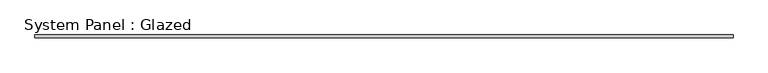
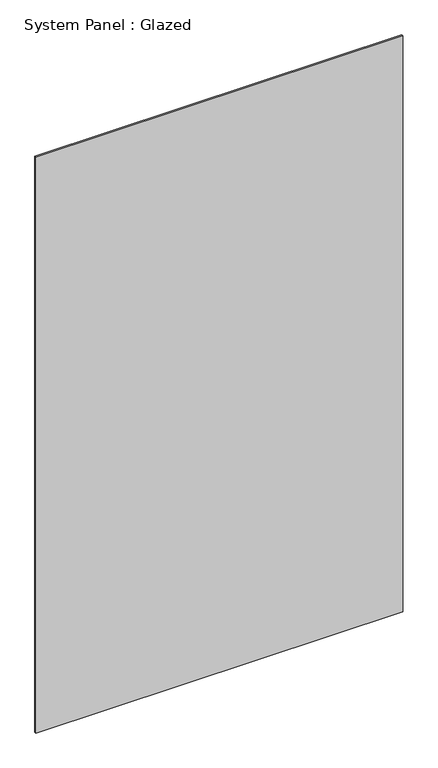
"""IFC4 building model written with IfcOpenShell, lengths in millimetres: plate geometry, System Panel : Glazed."""

from ifc_helpers import new_model, si_unit, origin, origin_with_axes, place, context, project, spatial, polyline, outline, extrude, source, transform, mapped, element, save


def system_panel_glazed_53b80dfb(model_context):
    return source(origin(), model_context, "Body", "SweptSolid", [
        extrude(outline(polyline([(708.3333334, 34.0), (-708.3333334, 34.0), (-708.3333334, 40.0), (708.3333334, 40.0), (708.3333334, 34.0)])), origin_with_axes(), (0.0, 0.0, 1.0), 2350.0),
    ])


if __name__ == "__main__":
    model = new_model("IFC4")
    model_context = context("Model", 3, world=origin())
    ifc_project = project(units=[si_unit("LENGTHUNIT", "METRE", prefix="MILLI")], contexts=[model_context])
    site = spatial("IfcSite", under=ifc_project)
    building = spatial("IfcBuilding", under=site)
    placement = place(None, origin())
    system_panel_glazed_shape = system_panel_glazed_53b80dfb(model_context)
    element("IfcPlate", 1, ObjectType="System Panel : Glazed", at=placement, inside=building, context=model_context, shape_type="MappedRepresentation", body=[
        mapped(system_panel_glazed_shape, transform((0.0, 0.0, 0.0), x_axis=(1.0, 0.0, 0.0), y_axis=(0.0, 1.0, 0.0), z_axis=(0.0, 0.0, 1.0))),
    ])
    save(model, "model.ifc")

# Revit data of these elements
# Type "System Panel : Glazed"
#   Construction Type Id = "GSP4R"
#   Analytic Construction = "1/8 in Pilkington single glazing"
#   Visual Light Transmittance = 0.9
#   Solar Heat Gain Coefficient = 0.86
#   Heat Transfer Coefficient (U) = 6.7069 W/(m²·K)
#   Define Thermal Properties by = 1
# Element 1 (IfcPlate, "System Panel : Glazed")
#   Materials on its faces: "Default New Material(6)"
# Materials
#   "Default New Material(6)": class "Generic", colour RGB 191 25 25, transparency 0.9, Cost = 0
